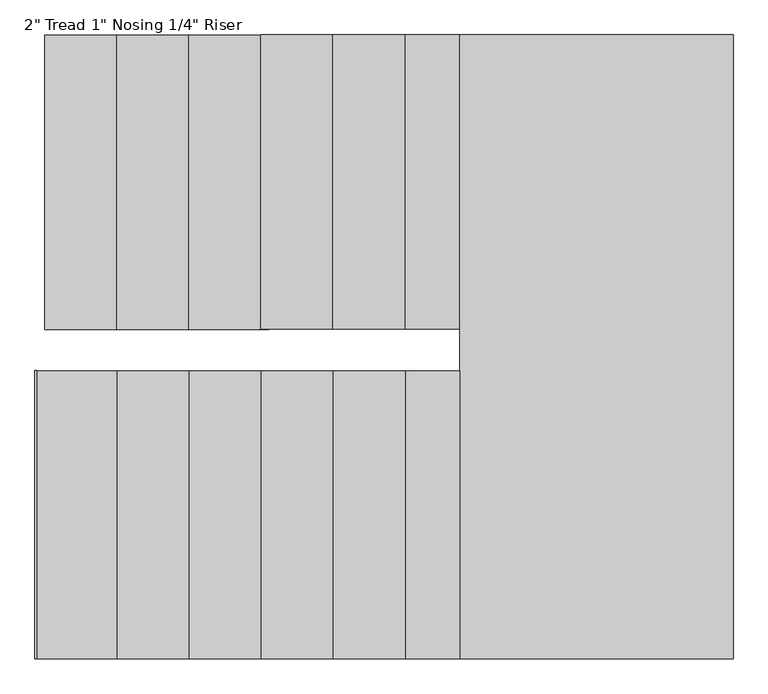
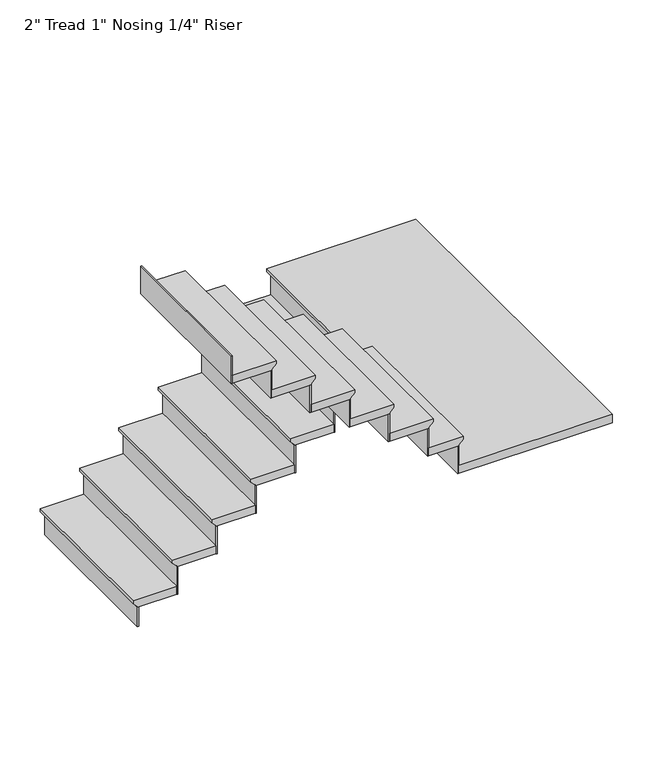
"""IFC4 building model written with IfcOpenShell, lengths in millimetres: stair flight geometry."""

from ifc_helpers import new_model, si_unit, origin, place, context, project, spatial, faceted_brep, source, transform, mapped, element, save


def stair_flight_b066332a(model_context):
    return source(origin(), model_context, "Body", "Brep", [
        faceted_brep([(-1022.6415352, -3861.2539367, 12951.8833333), (-1022.6415352, -3861.2539367, 12970.9333333), (-1022.6415352, -2926.4769687, 12970.9333333), (-1022.6415352, -2926.4769687, 12951.8833333), (-997.2415352, -3861.2539367, 12926.4833333), (-997.2415352, -2926.4769687, 12926.4833333), (-768.6415352, -3861.2539367, 12970.9333333), (-768.6415352, -2926.4769687, 12970.9333333), (-997.2415352, -2926.4769687, 12920.1333333), (-768.6415352, -2926.4769687, 12920.1333333), (-768.6415352, -3861.2539367, 12920.1333333), (-997.2415352, -3861.2539367, 12920.1333333)], [[[0, 1, 2, 3]], [[4, 0, 3, 5]], [[2, 1, 6, 7]], [[8, 9, 10, 11]], [[2, 7, 9, 8, 5, 3]], [[8, 11, 4, 5]], [[6, 1, 0, 4, 11, 10]], [[7, 6, 10, 9]]]),
        faceted_brep([(-997.2415352, -3861.2539367, 12920.1333333), (-997.2415352, -3861.2539367, 12801.6), (-990.8915352, -3861.2539367, 12801.6), (-990.8915352, -3861.2539367, 12920.1333333), (-997.2415352, -2926.4769687, 12920.1333333), (-990.8915352, -2926.4769687, 12920.1333333), (-990.8915352, -2926.4769687, 12801.6), (-997.2415352, -2926.4769687, 12801.6)], [[[0, 1, 2, 3]], [[4, 5, 6, 7]], [[1, 0, 4, 7]], [[2, 1, 7, 6]], [[3, 2, 6, 5]], [[0, 3, 5, 4]]]),
        faceted_brep([(-768.6415352, -3861.2539367, 13089.4666667), (-768.6415352, -3861.2539367, 12920.1333333), (-762.2915352, -3861.2539367, 12920.1333333), (-762.2915352, -3861.2539367, 13089.4666667), (-768.6415352, -2926.4769687, 13089.4666667), (-762.2915352, -2926.4769687, 13089.4666667), (-762.2915352, -2926.4769687, 12920.1333333), (-768.6415352, -2926.4769687, 12920.1333333)], [[[0, 1, 2, 3]], [[4, 5, 6, 7]], [[1, 0, 4, 7]], [[2, 1, 7, 6]], [[3, 2, 6, 5]], [[0, 3, 5, 4]]]),
        faceted_brep([(-794.0415352, -2926.4769687, 13140.2666667), (-794.0415352, -3861.2539367, 13140.2666667), (-540.0415352, -3861.2539367, 13140.2666667), (-540.0415352, -2926.4769687, 13140.2666667), (-768.6415352, -2926.4769687, 13089.4666667), (-540.0415352, -2926.4769687, 13089.4666667), (-540.0415352, -3861.2539367, 13089.4666667), (-768.6415352, -3861.2539367, 13089.4666667), (-768.6415352, -2926.4769687, 13095.8166667), (-794.0415352, -2926.4769687, 13121.2166667), (-768.6415352, -3861.2539367, 13095.8166667), (-794.0415352, -3861.2539367, 13121.2166667)], [[[0, 1, 2, 3]], [[4, 5, 6, 7]], [[0, 3, 5, 4, 8, 9]], [[4, 7, 10, 8]], [[2, 1, 11, 10, 7, 6]], [[3, 2, 6, 5]], [[11, 1, 0, 9]], [[10, 11, 9, 8]]]),
        faceted_brep([(-540.0415352, -3861.2539367, 13258.8), (-540.0415352, -3861.2539367, 13089.4666667), (-533.6915352, -3861.2539367, 13089.4666667), (-533.6915352, -3861.2539367, 13258.8), (-540.0415352, -2926.4769687, 13258.8), (-533.6915352, -2926.4769687, 13258.8), (-533.6915352, -2926.4769687, 13089.4666667), (-540.0415352, -2926.4769687, 13089.4666667)], [[[0, 1, 2, 3]], [[4, 5, 6, 7]], [[1, 0, 4, 7]], [[2, 1, 7, 6]], [[3, 2, 6, 5]], [[0, 3, 5, 4]]]),
        faceted_brep([(-565.4415352, -2926.4769687, 13309.6), (-565.4415352, -3861.2539367, 13309.6), (-311.4415352, -3861.2539367, 13309.6), (-311.4415352, -2926.4769687, 13309.6), (-540.0415352, -2926.4769687, 13258.8), (-311.4415352, -2926.4769687, 13258.8), (-311.4415352, -3861.2539367, 13258.8), (-540.0415352, -3861.2539367, 13258.8), (-540.0415352, -2926.4769687, 13265.15), (-565.4415352, -2926.4769687, 13290.55), (-540.0415352, -3861.2539367, 13265.15), (-565.4415352, -3861.2539367, 13290.55)], [[[0, 1, 2, 3]], [[4, 5, 6, 7]], [[0, 3, 5, 4, 8, 9]], [[4, 7, 10, 8]], [[2, 1, 11, 10, 7, 6]], [[3, 2, 6, 5]], [[11, 1, 0, 9]], [[10, 11, 9, 8]]]),
        faceted_brep([(-311.4415352, -3861.2539367, 13428.1333333), (-311.4415352, -3861.2539367, 13258.8), (-305.0915352, -3861.2539367, 13258.8), (-305.0915352, -3861.2539367, 13428.1333333), (-311.4415352, -2926.4769687, 13428.1333333), (-305.0915352, -2926.4769687, 13428.1333333), (-305.0915352, -2926.4769687, 13258.8), (-311.4415352, -2926.4769687, 13258.8)], [[[0, 1, 2, 3]], [[4, 5, 6, 7]], [[1, 0, 4, 7]], [[2, 1, 7, 6]], [[3, 2, 6, 5]], [[0, 3, 5, 4]]]),
        faceted_brep([(-336.8415352, -2926.4769687, 13478.9333333), (-336.8415352, -3861.2539367, 13478.9333333), (-82.8415352, -3861.2539367, 13478.9333333), (-82.8415352, -2926.4769687, 13478.9333333), (-311.4415352, -2926.4769687, 13428.1333333), (-82.8415352, -2926.4769687, 13428.1333333), (-82.8415352, -3861.2539367, 13428.1333333), (-311.4415352, -3861.2539367, 13428.1333333), (-311.4415352, -2926.4769687, 13434.4833333), (-336.8415352, -2926.4769687, 13459.8833333), (-311.4415352, -3861.2539367, 13434.4833333), (-336.8415352, -3861.2539367, 13459.8833333)], [[[0, 1, 2, 3]], [[4, 5, 6, 7]], [[0, 3, 5, 4, 8, 9]], [[4, 7, 10, 8]], [[2, 1, 11, 10, 7, 6]], [[3, 2, 6, 5]], [[11, 1, 0, 9]], [[10, 11, 9, 8]]]),
        faceted_brep([(-82.8415352, -3861.2539367, 13597.4666667), (-82.8415352, -3861.2539367, 13428.1333333), (-76.4915352, -3861.2539367, 13428.1333333), (-76.4915352, -3861.2539367, 13597.4666667), (-82.8415352, -2926.4769687, 13597.4666667), (-76.4915352, -2926.4769687, 13597.4666667), (-76.4915352, -2926.4769687, 13428.1333333), (-82.8415352, -2926.4769687, 13428.1333333)], [[[0, 1, 2, 3]], [[4, 5, 6, 7]], [[1, 0, 4, 7]], [[2, 1, 7, 6]], [[3, 2, 6, 5]], [[0, 3, 5, 4]]]),
        faceted_brep([(-108.2415352, -2926.4769687, 13648.2666667), (-108.2415352, -3861.2539367, 13648.2666667), (145.7584648, -3861.2539367, 13648.2666667), (145.7584648, -2926.4769687, 13648.2666667), (-82.8415352, -2926.4769687, 13597.4666667), (145.7584648, -2926.4769687, 13597.4666667), (145.7584648, -3861.2539367, 13597.4666667), (-82.8415352, -3861.2539367, 13597.4666667), (-82.8415352, -2926.4769687, 13603.8166667), (-108.2415352, -2926.4769687, 13629.2166667), (-82.8415352, -3861.2539367, 13603.8166667), (-108.2415352, -3861.2539367, 13629.2166667)], [[[0, 1, 2, 3]], [[4, 5, 6, 7]], [[0, 3, 5, 4, 8, 9]], [[4, 7, 10, 8]], [[2, 1, 11, 10, 7, 6]], [[3, 2, 6, 5]], [[11, 1, 0, 9]], [[10, 11, 9, 8]]]),
        faceted_brep([(145.7584648, -3861.2539367, 13766.8), (145.7584648, -3861.2539367, 13597.4666667), (152.1084648, -3861.2539367, 13597.4666667), (152.1084648, -3861.2539367, 13766.8), (145.7584648, -2926.4769687, 13766.8), (152.1084648, -2926.4769687, 13766.8), (152.1084648, -2926.4769687, 13597.4666667), (145.7584648, -2926.4769687, 13597.4666667)], [[[0, 1, 2, 3]], [[4, 5, 6, 7]], [[1, 0, 4, 7]], [[2, 1, 7, 6]], [[3, 2, 6, 5]], [[0, 3, 5, 4]]]),
        faceted_brep([(120.3584648, -2926.4769687, 13817.6), (120.3584648, -3861.2539367, 13817.6), (320.0221038, -3861.2539367, 13817.6), (320.0221038, -2926.4769687, 13817.6), (145.7584648, -2926.4769687, 13766.8), (320.0221038, -2926.4769687, 13766.8), (320.0221038, -3861.2539367, 13766.8), (145.7584648, -3861.2539367, 13766.8), (145.7584648, -2926.4769687, 13773.15), (120.3584648, -2926.4769687, 13798.55), (145.7584648, -3861.2539367, 13773.15), (120.3584648, -3861.2539367, 13798.55)], [[[0, 1, 2, 3]], [[4, 5, 6, 7]], [[0, 3, 5, 4, 8, 9]], [[4, 7, 10, 8]], [[2, 1, 11, 10, 7, 6]], [[3, 2, 6, 5]], [[11, 1, 0, 9]], [[10, 11, 9, 8]]]),
        faceted_brep([(320.0221038, -3861.2539367, 13936.1333333), (320.0221038, -3861.2539367, 13766.8), (326.3721038, -3861.2539367, 13766.8), (326.3721038, -3861.2539367, 13936.1333333), (320.0221038, -2926.4769687, 13936.1333333), (326.3721038, -2926.4769687, 13936.1333333), (326.3721038, -2926.4769687, 13766.8), (320.0221038, -2926.4769687, 13766.8)], [[[0, 1, 2, 3]], [[4, 5, 6, 7]], [[1, 0, 4, 7]], [[2, 1, 7, 6]], [[3, 2, 6, 5]], [[0, 3, 5, 4]]]),
        faceted_brep([(269.2221038, -4907.6769687, 13986.9333333), (1161.7584648, -4907.6769687, 13986.9333333), (1161.7584648, -2926.4769687, 13986.9333333), (294.6221038, -2926.4769687, 13986.9333333), (294.6221038, -3993.2769687, 13986.9333333), (269.2221038, -3993.2769687, 13986.9333333), (1161.7584648, -4907.6769687, 13936.1333333), (269.2221038, -4907.6769687, 13936.1333333), (269.2221038, -3993.2769687, 13936.1333333), (294.6221038, -3993.2769687, 13936.1333333), (294.6221038, -3861.2539367, 13936.1333333), (320.0221038, -3861.2539367, 13936.1333333), (320.0221038, -2926.4769687, 13936.1333333), (1161.7584648, -2926.4769687, 13936.1333333), (320.0221038, -2926.4769687, 13942.4833333), (294.6221038, -2926.4769687, 13967.8833333), (320.0221038, -3861.2539367, 13942.4833333), (294.6221038, -3861.2539367, 13967.8833333)], [[[0, 1, 2, 3, 4, 5]], [[6, 7, 8, 9, 10, 11, 12, 13]], [[1, 0, 7, 6]], [[2, 1, 6, 13]], [[3, 2, 13, 12, 14, 15]], [[12, 11, 16, 14]], [[11, 10, 17, 16]], [[4, 3, 15, 17, 10, 9]], [[5, 4, 9, 8]], [[0, 5, 8, 7]], [[15, 14, 16, 17]]]),
        faceted_brep([(269.2221038, -3993.2769687, 14105.4666667), (269.2221038, -3993.2769687, 13936.1333333), (262.8721038, -3993.2769687, 13936.1333333), (262.8721038, -3993.2769687, 14105.4666667), (269.2221038, -4907.6769687, 14105.4666667), (262.8721038, -4907.6769687, 14105.4666667), (262.8721038, -4907.6769687, 13936.1333333), (269.2221038, -4907.6769687, 13936.1333333)], [[[0, 1, 2, 3]], [[4, 5, 6, 7]], [[1, 0, 4, 7]], [[2, 1, 7, 6]], [[3, 2, 6, 5]], [[0, 3, 5, 4]]]),
        faceted_brep([(294.6221038, -4907.6769687, 14156.2666667), (294.6221038, -3993.2769687, 14156.2666667), (94.9584648, -3993.2769687, 14156.2666667), (94.9584648, -4907.6769687, 14156.2666667), (269.2221038, -4907.6769687, 14105.4666667), (94.9584648, -4907.6769687, 14105.4666667), (94.9584648, -3993.2769687, 14105.4666667), (269.2221038, -3993.2769687, 14105.4666667), (269.2221038, -4907.6769687, 14111.8166667), (294.6221038, -4907.6769687, 14137.2166667), (269.2221038, -3993.2769687, 14111.8166667), (294.6221038, -3993.2769687, 14137.2166667)], [[[0, 1, 2, 3]], [[4, 5, 6, 7]], [[0, 3, 5, 4, 8, 9]], [[4, 7, 10, 8]], [[2, 1, 11, 10, 7, 6]], [[3, 2, 6, 5]], [[11, 1, 0, 9]], [[10, 11, 9, 8]]]),
        faceted_brep([(94.9584648, -3993.2769687, 14274.8), (94.9584648, -3993.2769687, 14105.4666667), (88.6084648, -3993.2769687, 14105.4666667), (88.6084648, -3993.2769687, 14274.8), (94.9584648, -4907.6769687, 14274.8), (88.6084648, -4907.6769687, 14274.8), (88.6084648, -4907.6769687, 14105.4666667), (94.9584648, -4907.6769687, 14105.4666667)], [[[0, 1, 2, 3]], [[4, 5, 6, 7]], [[1, 0, 4, 7]], [[2, 1, 7, 6]], [[3, 2, 6, 5]], [[0, 3, 5, 4]]]),
        faceted_brep([(120.3584648, -4907.6769687, 14325.6), (120.3584648, -3993.2769687, 14325.6), (-133.6415352, -3993.2769687, 14325.6), (-133.6415352, -4907.6769687, 14325.6), (94.9584648, -4907.6769687, 14274.8), (-133.6415352, -4907.6769687, 14274.8), (-133.6415352, -3993.2769687, 14274.8), (94.9584648, -3993.2769687, 14274.8), (94.9584648, -4907.6769687, 14281.15), (120.3584648, -4907.6769687, 14306.55), (94.9584648, -3993.2769687, 14281.15), (120.3584648, -3993.2769687, 14306.55)], [[[0, 1, 2, 3]], [[4, 5, 6, 7]], [[0, 3, 5, 4, 8, 9]], [[4, 7, 10, 8]], [[2, 1, 11, 10, 7, 6]], [[3, 2, 6, 5]], [[11, 1, 0, 9]], [[10, 11, 9, 8]]]),
        faceted_brep([(-133.6415352, -3993.2769687, 14444.1333333), (-133.6415352, -3993.2769687, 14274.8), (-139.9915352, -3993.2769687, 14274.8), (-139.9915352, -3993.2769687, 14444.1333333), (-133.6415352, -4907.6769687, 14444.1333333), (-139.9915352, -4907.6769687, 14444.1333333), (-139.9915352, -4907.6769687, 14274.8), (-133.6415352, -4907.6769687, 14274.8)], [[[0, 1, 2, 3]], [[4, 5, 6, 7]], [[1, 0, 4, 7]], [[2, 1, 7, 6]], [[3, 2, 6, 5]], [[0, 3, 5, 4]]]),
        faceted_brep([(-108.2415352, -4907.6769687, 14494.9333333), (-108.2415352, -3993.2769687, 14494.9333333), (-362.2415352, -3993.2769687, 14494.9333333), (-362.2415352, -4907.6769687, 14494.9333333), (-133.6415352, -4907.6769687, 14444.1333333), (-362.2415352, -4907.6769687, 14444.1333333), (-362.2415352, -3993.2769687, 14444.1333333), (-133.6415352, -3993.2769687, 14444.1333333), (-133.6415352, -4907.6769687, 14450.4833333), (-108.2415352, -4907.6769687, 14475.8833333), (-133.6415352, -3993.2769687, 14450.4833333), (-108.2415352, -3993.2769687, 14475.8833333)], [[[0, 1, 2, 3]], [[4, 5, 6, 7]], [[0, 3, 5, 4, 8, 9]], [[4, 7, 10, 8]], [[2, 1, 11, 10, 7, 6]], [[3, 2, 6, 5]], [[11, 1, 0, 9]], [[10, 11, 9, 8]]]),
        faceted_brep([(-362.2415352, -3993.2769687, 14613.4666667), (-362.2415352, -3993.2769687, 14444.1333333), (-368.5915352, -3993.2769687, 14444.1333333), (-368.5915352, -3993.2769687, 14613.4666667), (-362.2415352, -4907.6769687, 14613.4666667), (-368.5915352, -4907.6769687, 14613.4666667), (-368.5915352, -4907.6769687, 14444.1333333), (-362.2415352, -4907.6769687, 14444.1333333)], [[[0, 1, 2, 3]], [[4, 5, 6, 7]], [[1, 0, 4, 7]], [[2, 1, 7, 6]], [[3, 2, 6, 5]], [[0, 3, 5, 4]]]),
        faceted_brep([(-336.8415352, -4907.6769687, 14664.2666667), (-336.8415352, -3993.2769687, 14664.2666667), (-590.8415352, -3993.2769687, 14664.2666667), (-590.8415352, -4907.6769687, 14664.2666667), (-362.2415352, -4907.6769687, 14613.4666667), (-590.8415352, -4907.6769687, 14613.4666667), (-590.8415352, -3993.2769687, 14613.4666667), (-362.2415352, -3993.2769687, 14613.4666667), (-362.2415352, -4907.6769687, 14619.8166667), (-336.8415352, -4907.6769687, 14645.2166667), (-362.2415352, -3993.2769687, 14619.8166667), (-336.8415352, -3993.2769687, 14645.2166667)], [[[0, 1, 2, 3]], [[4, 5, 6, 7]], [[0, 3, 5, 4, 8, 9]], [[4, 7, 10, 8]], [[2, 1, 11, 10, 7, 6]], [[3, 2, 6, 5]], [[11, 1, 0, 9]], [[10, 11, 9, 8]]]),
        faceted_brep([(-590.8415352, -3993.2769687, 14782.8), (-590.8415352, -3993.2769687, 14613.4666667), (-597.1915352, -3993.2769687, 14613.4666667), (-597.1915352, -3993.2769687, 14782.8), (-590.8415352, -4907.6769687, 14782.8), (-597.1915352, -4907.6769687, 14782.8), (-597.1915352, -4907.6769687, 14613.4666667), (-590.8415352, -4907.6769687, 14613.4666667)], [[[0, 1, 2, 3]], [[4, 5, 6, 7]], [[1, 0, 4, 7]], [[2, 1, 7, 6]], [[3, 2, 6, 5]], [[0, 3, 5, 4]]]),
        faceted_brep([(-565.4415352, -4907.6769687, 14833.6), (-565.4415352, -3993.2769687, 14833.6), (-819.4415352, -3993.2769687, 14833.6), (-819.4415352, -4907.6769687, 14833.6), (-590.8415352, -4907.6769687, 14782.8), (-819.4415352, -4907.6769687, 14782.8), (-819.4415352, -3993.2769687, 14782.8), (-590.8415352, -3993.2769687, 14782.8), (-590.8415352, -4907.6769687, 14789.15), (-565.4415352, -4907.6769687, 14814.55), (-590.8415352, -3993.2769687, 14789.15), (-565.4415352, -3993.2769687, 14814.55)], [[[0, 1, 2, 3]], [[4, 5, 6, 7]], [[0, 3, 5, 4, 8, 9]], [[4, 7, 10, 8]], [[2, 1, 11, 10, 7, 6]], [[3, 2, 6, 5]], [[11, 1, 0, 9]], [[10, 11, 9, 8]]]),
        faceted_brep([(-819.4415352, -3993.2769687, 14952.1333333), (-819.4415352, -3993.2769687, 14782.8), (-825.7915352, -3993.2769687, 14782.8), (-825.7915352, -3993.2769687, 14952.1333333), (-819.4415352, -4907.6769687, 14952.1333333), (-825.7915352, -4907.6769687, 14952.1333333), (-825.7915352, -4907.6769687, 14782.8), (-819.4415352, -4907.6769687, 14782.8)], [[[0, 1, 2, 3]], [[4, 5, 6, 7]], [[1, 0, 4, 7]], [[2, 1, 7, 6]], [[3, 2, 6, 5]], [[0, 3, 5, 4]]]),
        faceted_brep([(-1048.0415352, -3993.2769687, 15121.4666667), (-1048.0415352, -3993.2769687, 14952.1333333), (-1054.3915352, -3993.2769687, 14952.1333333), (-1054.3915352, -3993.2769687, 15121.4666667), (-1048.0415352, -4907.6769687, 15121.4666667), (-1054.3915352, -4907.6769687, 15121.4666667), (-1054.3915352, -4907.6769687, 14952.1333333), (-1048.0415352, -4907.6769687, 14952.1333333)], [[[0, 1, 2, 3]], [[4, 5, 6, 7]], [[1, 0, 4, 7]], [[2, 1, 7, 6]], [[3, 2, 6, 5]], [[0, 3, 5, 4]]]),
        faceted_brep([(-794.0415352, -4907.6769687, 15002.9333333), (-794.0415352, -3993.2769687, 15002.9333333), (-1048.0415352, -3993.2769687, 15002.9333333), (-1048.0415352, -4907.6769687, 15002.9333333), (-819.4415352, -4907.6769687, 14952.1333333), (-1048.0415352, -4907.6769687, 14952.1333333), (-1048.0415352, -3993.2769687, 14952.1333333), (-819.4415352, -3993.2769687, 14952.1333333), (-819.4415352, -4907.6769687, 14958.4833333), (-794.0415352, -4907.6769687, 14983.8833333), (-819.4415352, -3993.2769687, 14958.4833333), (-794.0415352, -3993.2769687, 14983.8833333)], [[[0, 1, 2, 3]], [[4, 5, 6, 7]], [[0, 3, 5, 4, 8, 9]], [[4, 7, 10, 8]], [[2, 1, 11, 10, 7, 6]], [[3, 2, 6, 5]], [[11, 1, 0, 9]], [[10, 11, 9, 8]]]),
    ])


if __name__ == "__main__":
    model = new_model("IFC4")
    model_context = context("Model", 3, world=origin())
    ifc_project = project(units=[si_unit("LENGTHUNIT", "METRE", prefix="MILLI")], contexts=[model_context])
    site = spatial("IfcSite", under=ifc_project)
    building = spatial("IfcBuilding", under=site)
    placement = place(None, origin())
    stair_flight_shape = stair_flight_b066332a(model_context)
    element("IfcStairFlight", 1, ObjectType="2\" Tread 1\" Nosing 1/4\" Riser", at=placement, inside=building, context=model_context, shape_type="MappedRepresentation", body=[
        mapped(stair_flight_shape, transform((0.0, 0.0, 0.0), x_axis=(1.0, 0.0, 0.0), y_axis=(0.0, 1.0, 0.0), z_axis=(0.0, 0.0, 1.0))),
    ])
    save(model, "model.ifc")
